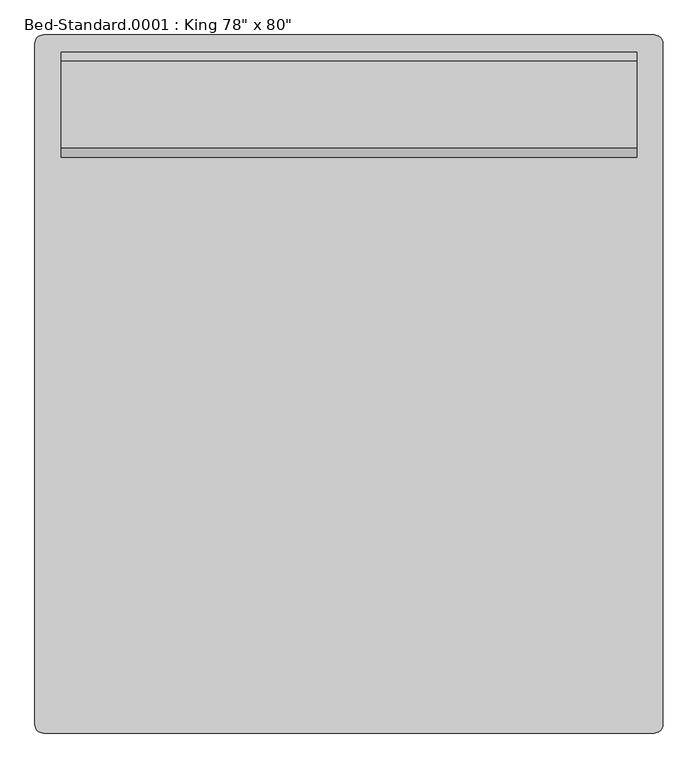
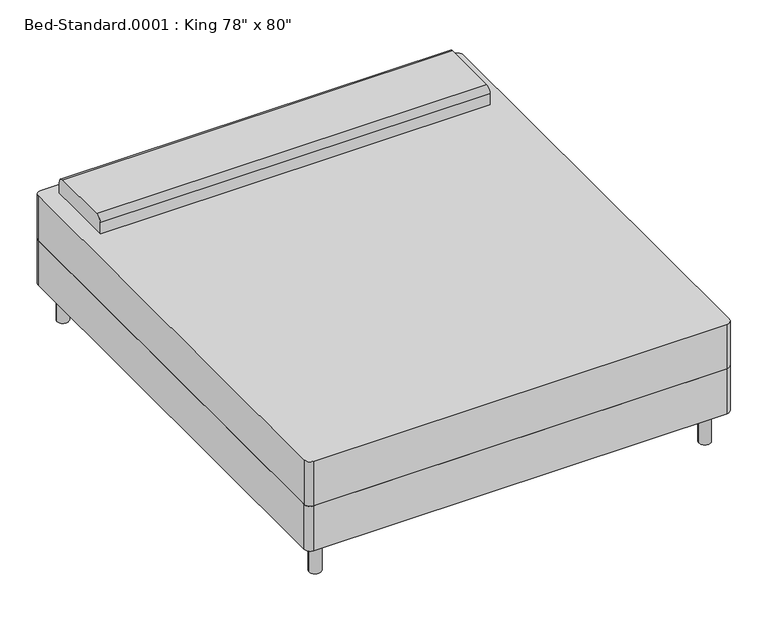
"""IFC4 building model written with IfcOpenShell, lengths in millimetres: furniture geometry."""

from ifc_helpers import new_model, si_unit, point, frame, frame_2d, origin, origin_with_axes, place, context, project, spatial, polyline, circle_curve, trimmed, segment, composite_curve, outline, extrude, source, transform, mapped, element, save


def furniture_a8794613(model_context):
    return source(origin(), model_context, "Body", "SweptSolid", [
        extrude(outline(composite_curve([segment(polyline([(-642.9114754, -1036.195082), (-642.9114754, 945.004918)]), True, "CONTINUOUS"), segment(trimmed(circle_curve(frame_2d((-617.5114754, 945.004918)), 25.4), [point((-642.9114754, 945.004918))], [point((-617.5114754, 970.404918))], False, "CARTESIAN"), True, "CONTINUOUS"), segment(polyline([(-617.5114754, 970.404918), (1160.4885246, 970.404918)]), True, "CONTINUOUS"), segment(trimmed(circle_curve(frame_2d((1160.4885246, 945.004918)), 25.4), [point((1160.4885246, 970.404918))], [point((1185.8885246, 945.004918))], False, "CARTESIAN"), True, "CONTINUOUS"), segment(polyline([(1185.8885246, 945.004918), (1185.8885246, -1036.195082)]), True, "CONTINUOUS"), segment(trimmed(circle_curve(frame_2d((1160.4885246, -1036.195082)), 25.4), [point((1185.8885246, -1036.195082))], [point((1160.4885246, -1061.595082))], False, "CARTESIAN"), True, "CONTINUOUS"), segment(polyline([(1160.4885246, -1061.595082), (-617.5114754, -1061.595082)]), True, "CONTINUOUS"), segment(trimmed(circle_curve(frame_2d((-617.5114754, -1036.195082)), 25.4), [point((-617.5114754, -1061.595082))], [point((-642.9114754, -1036.195082))], False, "CARTESIAN"), True, "CONTINUOUS")], self_intersect=False)), frame((0.0, 0.0, 152.4), z_axis=(0.0, 0.0, 1.0), x_axis=(1.0, 0.0, 0.0)), (0.0, 0.0, 1.0), 203.2),
        extrude(outline(composite_curve([segment(polyline([(614.804918, 558.8), (614.804918, 609.6)]), True, "CONTINUOUS"), segment(trimmed(circle_curve(frame_2d((640.204918, 609.6)), 25.4), [point((614.804918, 609.6))], [point((640.204918, 635.0))], False, "CARTESIAN"), True, "CONTINUOUS"), segment(polyline([(640.204918, 635.0), (894.204918, 635.0)]), True, "CONTINUOUS"), segment(trimmed(circle_curve(frame_2d((894.204918, 609.6)), 25.4), [point((894.204918, 635.0))], [point((919.604918, 609.6))], False, "CARTESIAN"), True, "CONTINUOUS"), segment(polyline([(919.604918, 609.6), (919.604918, 558.8), (614.804918, 558.8)]), True, "CONTINUOUS")], self_intersect=False)), frame((-566.7114754, 0.0, 0.0), z_axis=(1.0, 0.0, 0.0), x_axis=(0.0, 1.0, 0.0)), (0.0, 0.0, 1.0), 1676.4),
        extrude(outline(composite_curve([segment(trimmed(circle_curve(frame_2d((-566.7114754, 894.204918)), 25.4), [point((-592.1114754, 894.204918))], [point((-541.3114754, 894.204918))], False, "CARTESIAN"), True, "CONTINUOUS"), segment(trimmed(circle_curve(frame_2d((-566.7114754, 894.204918)), 25.4), [point((-541.3114754, 894.204918))], [point((-592.1114754, 894.204918))], False, "CARTESIAN"), True, "CONTINUOUS")], self_intersect=False)), origin_with_axes(), (0.0, 0.0, 1.0), 152.4),
        extrude(outline(composite_curve([segment(trimmed(circle_curve(frame_2d((1109.6885246, 894.204918)), 25.4), [point((1084.2885246, 894.204918))], [point((1135.0885246, 894.204918))], False, "CARTESIAN"), True, "CONTINUOUS"), segment(trimmed(circle_curve(frame_2d((1109.6885246, 894.204918)), 25.4), [point((1135.0885246, 894.204918))], [point((1084.2885246, 894.204918))], False, "CARTESIAN"), True, "CONTINUOUS")], self_intersect=False)), origin_with_axes(), (0.0, 0.0, 1.0), 152.4),
        extrude(outline(composite_curve([segment(trimmed(circle_curve(frame_2d((1109.6885246, -985.395082)), 25.4), [point((1084.2885246, -985.395082))], [point((1135.0885246, -985.395082))], False, "CARTESIAN"), True, "CONTINUOUS"), segment(trimmed(circle_curve(frame_2d((1109.6885246, -985.395082)), 25.4), [point((1135.0885246, -985.395082))], [point((1084.2885246, -985.395082))], False, "CARTESIAN"), True, "CONTINUOUS")], self_intersect=False)), origin_with_axes(), (0.0, 0.0, 1.0), 152.4),
        extrude(outline(composite_curve([segment(trimmed(circle_curve(frame_2d((-566.7114754, -985.395082)), 25.4), [point((-592.1114754, -985.395082))], [point((-541.3114754, -985.395082))], False, "CARTESIAN"), True, "CONTINUOUS"), segment(trimmed(circle_curve(frame_2d((-566.7114754, -985.395082)), 25.4), [point((-541.3114754, -985.395082))], [point((-592.1114754, -985.395082))], False, "CARTESIAN"), True, "CONTINUOUS")], self_intersect=False)), origin_with_axes(), (0.0, 0.0, 1.0), 152.4),
        extrude(outline(composite_curve([segment(polyline([(-617.5114754, 970.404918), (1160.4885246, 970.404918)]), True, "CONTINUOUS"), segment(trimmed(circle_curve(frame_2d((1160.4885246, 945.004918)), 25.4), [point((1160.4885246, 970.404918))], [point((1185.8885246, 945.004918))], False, "CARTESIAN"), True, "CONTINUOUS"), segment(polyline([(1185.8885246, 945.004918), (1185.8885246, -1036.195082)]), True, "CONTINUOUS"), segment(trimmed(circle_curve(frame_2d((1160.4885246, -1036.195082)), 25.4), [point((1185.8885246, -1036.195082))], [point((1160.4885246, -1061.595082))], False, "CARTESIAN"), True, "CONTINUOUS"), segment(polyline([(1160.4885246, -1061.595082), (-617.5114754, -1061.595082)]), True, "CONTINUOUS"), segment(trimmed(circle_curve(frame_2d((-617.5114754, -1036.195082)), 25.4), [point((-617.5114754, -1061.595082))], [point((-642.9114754, -1036.195082))], False, "CARTESIAN"), True, "CONTINUOUS"), segment(polyline([(-642.9114754, -1036.195082), (-642.9114754, 945.004918)]), True, "CONTINUOUS"), segment(trimmed(circle_curve(frame_2d((-617.5114754, 945.004918)), 25.4), [point((-642.9114754, 945.004918))], [point((-617.5114754, 970.404918))], False, "CARTESIAN"), True, "CONTINUOUS")], self_intersect=False)), frame((0.0, 0.0, 355.6), z_axis=(0.0, 0.0, 1.0), x_axis=(1.0, 0.0, 0.0)), (0.0, 0.0, 1.0), 203.2),
    ])


if __name__ == "__main__":
    model = new_model("IFC4")
    model_context = context("Model", 3, world=origin())
    ifc_project = project(units=[si_unit("LENGTHUNIT", "METRE", prefix="MILLI")], contexts=[model_context])
    site = spatial("IfcSite", under=ifc_project)
    building = spatial("IfcBuilding", under=site)
    placement = place(None, origin())
    furniture_shape = furniture_a8794613(model_context)
    element("IfcFurniture", 1, ObjectType="Bed-Standard.0001 : King 78\" x 80\"", at=placement, inside=building, context=model_context, shape_type="MappedRepresentation", body=[
        mapped(furniture_shape, transform((0.0, 0.0, 0.0), x_axis=(1.0, 0.0, 0.0), y_axis=(0.0, 1.0, 0.0), z_axis=(0.0, 0.0, 1.0))),
    ])
    save(model, "model.ifc")

# Revit data of these elements
# Type "Bed-Standard.0001 : King 78\" x 80\""
#   Assembly Code = "E2020200"
#   Length = 6' - 8"
#   Width = 6' - 0"
#   Leg Material = Steel, Chrome Plated
#   Mattress Material = Linen, White
#   Default Elevation = 0
# Element 1 (IfcFurniture, "Bed-Standard.0001 : King 78\" x 80\"")
#   Materials on its faces: "Linen, White", "Steel, Chrome Plated"
# Materials
#   "Steel, Chrome Plated": class "Metal", colour RGB 17 17 17, transparency 0, Description = "Chromiuim plated steel", Cost = 0
#   "Linen, White": class "Textile", colour RGB 247 247 239, transparency 0, Description = "Linen, white", Cost = 0
